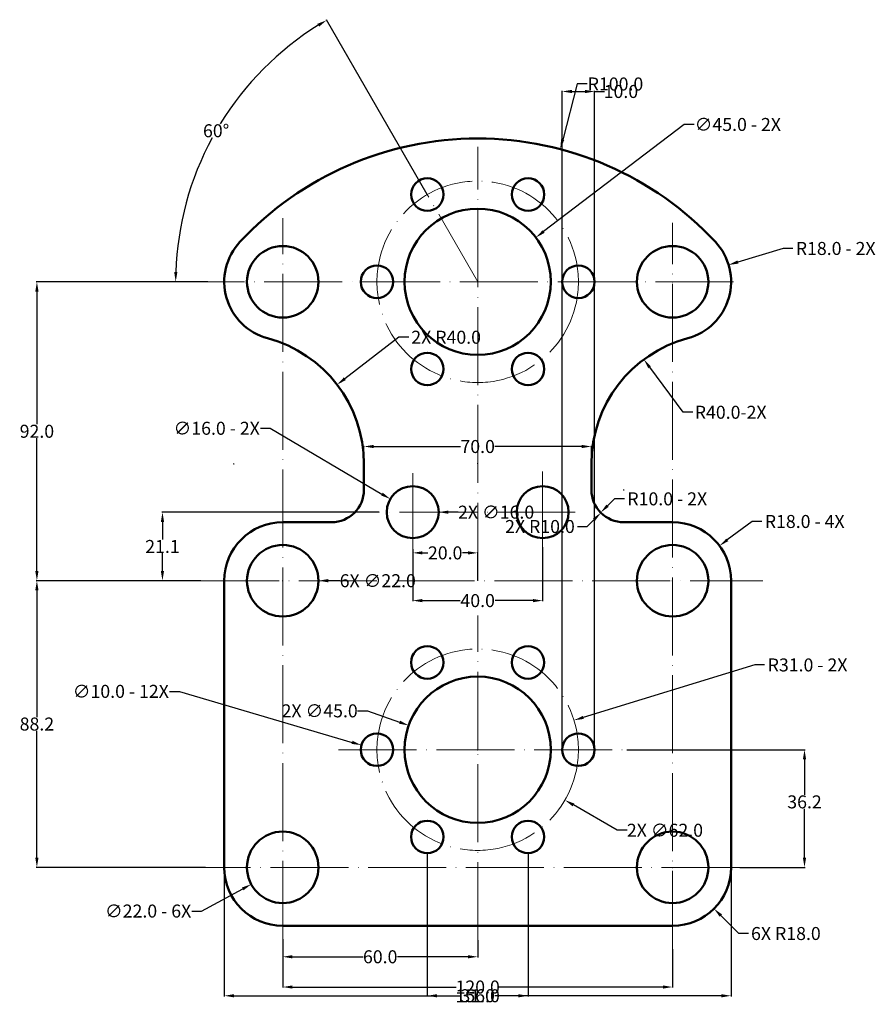
# Model space of a CAD drawing. Units: inches. Extents: x 135 to 399, y 77 to 380.
import ezdxf

# ---------------------------------------------------------------- set-up
doc = ezdxf.new("R2010")
doc.units = ezdxf.units.IN
doc.header["$MEASUREMENT"] = 0
doc.linetypes.add('ACAD_ISO04W100', pattern=[30, 24, -3, 0, -3])
for name, color, linetype, lineweight in [('M-CNTR', 4, 'ACAD_ISO04W100', 18), ('M-DIMS', 2, 'Continuous', 25), ('M-OUTL', 7, 'Continuous', 50)]:
    doc.layers.add(name, color=color, linetype=linetype, lineweight=lineweight)
doc.styles.get("Standard").update_dxf_attribs({"font": 'arial.ttf'})
doc.dimstyles.get("Standard").update_dxf_attribs({"dimtxt": 4, "dimasz": 3, "dimexe": 0.18, "dimexo": 0.0625, "dimgap": 0.09, "dimtad": 0, "dimtih": 1, "dimtoh": 1, "dimdec": 1, "dimzin": 0, "dimdsep": 46, "dimtxsty": 'Standard', "dimcen": 0.09, "dimclrd": 1, "dimclre": 1, "dimadec": 0, "dimazin": 0, "dimtfac": 1, "dimtdec": 1, "dimtofl": 0, "dimtmove": 0, "dimatfit": 3, "dimfxl": 1, "dimtolj": 1, "dimtzin": 0, "dimarcsym": 0})

# ---------------------------------------------------------------- blocks, each defined once
blk = doc.blocks.new('*U1')
blk.add_circle((0, 0), 5)
blk = doc.blocks.new('*U2')
at = {"layer": 'M-OUTL', "color": 0, "linetype": 'ByBlock', "lineweight": -2, "transparency": 16777216}
for p, rotation in [((163.06, 105.92), 120), ((194.06, 105.92), 59.99999999999999), ((147.56, 79.07), 180), ((163.06, 52.23), 239.9999999999999), ((194.06, 52.23), 299.9999999999999)]:
    blk.add_blockref('*U1', p, dxfattribs=dict(at, rotation=rotation))
blk.add_blockref('*U1', (209.56, 79.07), dxfattribs=at)
blk = doc.blocks.new('*D3')
at = {"layer": 'Defpoints', "color": 0, "transparency": 16777216}
for p in [(322.16, 155.02), (356.94, 118.82), (376.93, 118.82)]:
    blk.add_point(p, dxfattribs=at)
at = {"layer": 'M-DIMS', "color": 0, "lineweight": -2, "transparency": 16777216}
for p, q in [((322.22, 155.02), (377.11, 155.02)), ((376.93, 152.02), (376.93, 141.1)), ((376.93, 121.82), (376.93, 136.83)), ((357, 118.82), (377.11, 118.82))]:
    blk.add_line(p, q, dxfattribs=at)
at = {"layer": 'M-DIMS', "color": 0, "transparency": 16777216}
for points in [[(376.43, 152.02), (377.43, 152.02), (376.93, 155.02)], [(376.43, 121.82), (377.43, 121.82), (376.93, 118.82)]]:
    blk.add_solid(points, dxfattribs=at)
at = {"layer": 'M-DIMS', "color": 0, "transparency": 16777216, "insert": (376.93, 138.97), "char_height": 4, "attachment_point": 5}
blk.add_mtext('\\A1;36.2', dxfattribs=at)
blk = doc.blocks.new('*D4')
at = {"layer": 'Defpoints', "color": 0, "transparency": 16777216}
for p in [(216.34, 96.82), (276.34, 96.43), (216.34, 91.3)]:
    blk.add_point(p, dxfattribs=at)
at = {"layer": 'M-DIMS', "color": 0, "lineweight": -2, "transparency": 16777216}
for p, q in [((216.34, 96.76), (216.34, 91.12)), ((276.34, 96.37), (276.34, 91.12)), ((219.34, 91.3), (241.05, 91.3)), ((273.34, 91.3), (251.63, 91.3))]:
    blk.add_line(p, q, dxfattribs=at)
at = {"layer": 'M-DIMS', "color": 0, "transparency": 16777216}
for points in [[(219.34, 91.8), (219.34, 90.8), (216.34, 91.3)], [(273.34, 91.8), (273.34, 90.8), (276.34, 91.3)]]:
    blk.add_solid(points, dxfattribs=at)
at = {"layer": 'M-DIMS', "color": 0, "transparency": 16777216, "insert": (246.34, 91.3), "char_height": 4, "attachment_point": 5}
blk.add_mtext('\\A1;60.0', dxfattribs=at)
blk = doc.blocks.new('*D5')
at = {"layer": 'Defpoints', "color": 0, "transparency": 16777216}
for p in [(216.34, 96.82), (336.34, 93.75), (216.34, 81.99)]:
    blk.add_point(p, dxfattribs=at)
at = {"layer": 'M-DIMS', "color": 0, "lineweight": -2, "transparency": 16777216}
for p, q in [((216.34, 96.76), (216.34, 81.81)), ((336.34, 93.68), (336.34, 81.81)), ((219.34, 81.99), (269.69, 81.99)), ((333.34, 81.99), (282.98, 81.99))]:
    blk.add_line(p, q, dxfattribs=at)
at = {"layer": 'M-DIMS', "color": 0, "transparency": 16777216}
for points in [[(219.34, 82.49), (219.34, 81.49), (216.34, 81.99)], [(333.34, 82.49), (333.34, 81.49), (336.34, 81.99)]]:
    blk.add_solid(points, dxfattribs=at)
at = {"layer": 'M-DIMS', "color": 0, "transparency": 16777216, "insert": (276.34, 81.99), "char_height": 4, "attachment_point": 5}
blk.add_mtext('\\A1;120.0', dxfattribs=at)
blk = doc.blocks.new('*D6')
at = {"layer": 'Defpoints', "color": 0, "transparency": 16777216}
for p in [(226.02, 124.04), (206.65, 113.61)]:
    blk.add_point(p, dxfattribs=at)
at = {"layer": 'M-DIMS', "color": 0, "lineweight": -2, "transparency": 16777216}
for p, q in [((216.25, 118.82), (216.43, 118.82)), ((216.34, 118.73), (216.34, 118.91)), ((191.38, 105.37), (204.01, 112.18)), ((188.38, 105.37), (191.38, 105.37))]:
    blk.add_line(p, q, dxfattribs=at)
at = {"layer": 'M-DIMS', "color": 0, "transparency": 16777216}
blk.add_solid([(203.78, 112.62), (204.25, 111.74), (206.65, 113.61)], dxfattribs=at)
at = {"layer": 'M-DIMS', "color": 0, "transparency": 16777216, "insert": (174.91, 105.37), "char_height": 4, "attachment_point": 5}
blk.add_mtext('\\A1;∅22.0 - 6X', dxfattribs=at)
blk = doc.blocks.new('*D7')
at = {"layer": 'Defpoints', "color": 0, "transparency": 16777216}
for p in [(305.98, 164.09), (276.34, 155.02)]:
    blk.add_point(p, dxfattribs=at)
at = {"layer": 'M-DIMS', "color": 0, "lineweight": -2, "transparency": 16777216}
for p, q in [((361.66, 181.11), (308.85, 164.97)), ((364.66, 181.11), (361.66, 181.11)), ((276.25, 155.02), (276.43, 155.02)), ((276.34, 154.93), (276.34, 155.11))]:
    blk.add_line(p, q, dxfattribs=at)
at = {"layer": 'M-DIMS', "color": 0, "transparency": 16777216}
blk.add_solid([(308.71, 165.44), (309, 164.49), (305.98, 164.09)], dxfattribs=at)
at = {"layer": 'M-DIMS', "color": 0, "transparency": 16777216, "insert": (377.87, 181.11), "char_height": 4, "attachment_point": 5}
blk.add_mtext('\\A1;R31.0 - 2X', dxfattribs=at)
blk = doc.blocks.new('*D8')
at = {"layer": 'Defpoints', "color": 0, "transparency": 16777216}
for p in [(240.54, 156.44), (250.13, 153.61)]:
    blk.add_point(p, dxfattribs=at)
at = {"layer": 'M-DIMS', "color": 0, "lineweight": -2, "transparency": 16777216}
for p, q in [((181.54, 172.98), (184.54, 172.98)), ((184.54, 172.98), (237.67, 157.29)), ((245.25, 155.02), (245.43, 155.02)), ((245.34, 154.93), (245.34, 155.11))]:
    blk.add_line(p, q, dxfattribs=at)
at = {"layer": 'M-DIMS', "color": 0, "transparency": 16777216}
blk.add_solid([(237.81, 157.77), (237.52, 156.81), (240.54, 156.44)], dxfattribs=at)
at = {"layer": 'M-DIMS', "color": 0, "transparency": 16777216, "insert": (166.51, 172.98), "char_height": 4, "attachment_point": 5}
blk.add_mtext('\\A1;∅10.0 - 12X', dxfattribs=at)
blk = doc.blocks.new('*D9')
at = {"layer": 'Defpoints', "color": 0, "transparency": 16777216}
for p in [(191.21, 207.02), (140.68, 118.82), (192.68, 118.82)]:
    blk.add_point(p, dxfattribs=at)
at = {"layer": 'M-DIMS', "color": 0, "lineweight": -2, "transparency": 16777216}
for p, q in [((191.15, 207.02), (140.5, 207.02)), ((140.68, 204.02), (140.68, 165.06)), ((140.68, 121.82), (140.68, 160.79)), ((192.62, 118.82), (140.5, 118.82))]:
    blk.add_line(p, q, dxfattribs=at)
at = {"layer": 'M-DIMS', "color": 0, "transparency": 16777216}
for points in [[(140.18, 204.02), (141.18, 204.02), (140.68, 207.02)], [(140.18, 121.82), (141.18, 121.82), (140.68, 118.82)]]:
    blk.add_solid(points, dxfattribs=at)
at = {"layer": 'M-DIMS', "color": 0, "transparency": 16777216, "insert": (140.68, 162.92), "char_height": 4, "attachment_point": 5}
blk.add_mtext('\\A1;88.2', dxfattribs=at)
blk = doc.blocks.new('*D10')
at = {"layer": 'Defpoints', "color": 0, "transparency": 16777216}
for p in [(179.32, 228.12), (246.09, 228.12), (191.21, 207.02)]:
    blk.add_point(p, dxfattribs=at)
at = {"layer": 'M-DIMS', "color": 0, "lineweight": -2, "transparency": 16777216}
for p, q in [((246.02, 228.12), (179.14, 228.12)), ((179.32, 225.12), (179.32, 219.67)), ((179.32, 210.02), (179.32, 215.48)), ((191.15, 207.02), (179.14, 207.02))]:
    blk.add_line(p, q, dxfattribs=at)
at = {"layer": 'M-DIMS', "color": 0, "transparency": 16777216}
for points in [[(178.82, 225.12), (179.82, 225.12), (179.32, 228.12)], [(178.82, 210.02), (179.82, 210.02), (179.32, 207.02)]]:
    blk.add_solid(points, dxfattribs=at)
at = {"layer": 'M-DIMS', "color": 0, "transparency": 16777216, "insert": (179.32, 217.57), "char_height": 4, "attachment_point": 5}
blk.add_mtext('\\A1;21.1', dxfattribs=at)
blk = doc.blocks.new('*D11')
at = {"layer": 'Defpoints', "color": 0, "transparency": 16777216}
for p in [(256.34, 216.79), (296.34, 217.44), (296.34, 200.91)]:
    blk.add_point(p, dxfattribs=at)
at = {"layer": 'M-DIMS', "color": 0, "lineweight": -2, "transparency": 16777216}
for p, q in [((256.34, 216.73), (256.34, 200.73)), ((296.34, 217.38), (296.34, 200.73)), ((259.34, 200.91), (270.98, 200.91)), ((293.34, 200.91), (281.7, 200.91))]:
    blk.add_line(p, q, dxfattribs=at)
at = {"layer": 'M-DIMS', "color": 0, "transparency": 16777216}
for points in [[(259.34, 201.41), (259.34, 200.41), (256.34, 200.91)], [(293.34, 201.41), (293.34, 200.41), (296.34, 200.91)]]:
    blk.add_solid(points, dxfattribs=at)
at = {"layer": 'M-DIMS', "color": 0, "transparency": 16777216, "insert": (276.34, 200.91), "char_height": 4, "attachment_point": 5}
blk.add_mtext('\\A1;40.0', dxfattribs=at)
blk = doc.blocks.new('*D12')
at = {"layer": 'Defpoints', "color": 0, "transparency": 16777216}
for p in [(249.44, 232.18), (263.23, 224.07)]:
    blk.add_point(p, dxfattribs=at)
at = {"layer": 'M-DIMS', "color": 0, "lineweight": -2, "transparency": 16777216}
for p, q in [((209.49, 253.94), (212.49, 253.94)), ((212.49, 253.94), (246.86, 233.71)), ((256.25, 228.12), (256.43, 228.12)), ((256.34, 228.03), (256.34, 228.21))]:
    blk.add_line(p, q, dxfattribs=at)
at = {"layer": 'M-DIMS', "color": 0, "transparency": 16777216}
blk.add_solid([(247.11, 234.14), (246.6, 233.27), (249.44, 232.18)], dxfattribs=at)
at = {"layer": 'M-DIMS', "color": 0, "transparency": 16777216, "insert": (196.02, 253.94), "char_height": 4, "attachment_point": 5}
blk.add_mtext('\\A1;∅16.0 - 2X', dxfattribs=at)
blk = doc.blocks.new('*D13')
at = {"layer": 'Defpoints', "color": 0, "transparency": 16777216}
for p in [(256.34, 216.79), (276.34, 215.6), (276.34, 207.02)]:
    blk.add_point(p, dxfattribs=at)
at = {"layer": 'M-DIMS', "color": 0, "lineweight": -2, "transparency": 16777216}
for p, q in [((256.34, 216.73), (256.34, 215.42)), ((259.34, 215.6), (261.03, 215.6)), ((273.34, 215.6), (271.65, 215.6)), ((276.34, 207.09), (276.34, 215.78))]:
    blk.add_line(p, q, dxfattribs=at)
at = {"layer": 'M-DIMS', "color": 0, "transparency": 16777216}
for points in [[(259.34, 216.1), (259.34, 215.1), (256.34, 215.6)], [(273.34, 216.1), (273.34, 215.1), (276.34, 215.6)]]:
    blk.add_solid(points, dxfattribs=at)
at = {"layer": 'M-DIMS', "color": 0, "transparency": 16777216, "insert": (266.34, 215.6), "char_height": 4, "attachment_point": 5}
blk.add_mtext('\\A1;20.0', dxfattribs=at)
blk = doc.blocks.new('*U14')
blk.add_circle((0, 0), 5)
blk = doc.blocks.new('*U15')
at = {"layer": 'M-OUTL', "color": 0, "linetype": 'ByBlock', "lineweight": -2, "transparency": 16777216}
for p, rotation in [((260.84, 325.87), 120), ((291.84, 325.87), 59.99999999999999), ((245.34, 299.02), 180), ((260.84, 272.18), 239.9999999999999), ((291.84, 272.18), 299.9999999999999)]:
    blk.add_blockref('*U14', p, dxfattribs=dict(at, rotation=rotation))
blk.add_blockref('*U14', (307.34, 299.02), dxfattribs=at)
blk = doc.blocks.new('*D16')
at = {"layer": 'Defpoints', "color": 0, "transparency": 16777216}
for p in [(205.13, 358.77), (260.84, 325.87), (193.34, 299.02), (276.34, 299.02), (355.06, 299.02)]:
    blk.add_point(p, dxfattribs=at)
at = {"layer": 'M-DIMS', "color": 0, "lineweight": -2, "transparency": 16777216}
for p, q in [((260.81, 325.93), (229.77, 379.68)), ((193.27, 299.02), (183.21, 299.02))]:
    blk.add_line(p, q, dxfattribs=at)
for start, end in [(121.8493, 148.4703), (151.5064, 178.1507)]:
    blk.add_arc((276.34, 299.02), 92.95, start, end, dxfattribs=at)
at = {"layer": 'M-DIMS', "color": 0, "transparency": 16777216}
for points in [[(227.03, 378.41), (227.55, 377.55), (229.86, 379.52)], [(183.93, 302.02), (182.94, 302.03), (183.39, 299.02)]]:
    blk.add_solid(points, dxfattribs=at)
at = {"layer": 'M-DIMS', "color": 0, "transparency": 16777216, "insert": (195.84, 345.5), "char_height": 4, "attachment_point": 5}
blk.add_mtext('\\A1;60°', dxfattribs=at)
blk = doc.blocks.new('*D17')
at = {"layer": 'Defpoints', "color": 0, "transparency": 16777216}
for p in [(301.74, 339.85), (276.34, 243.13)]:
    blk.add_point(p, dxfattribs=at)
at = {"layer": 'M-DIMS', "color": 0, "lineweight": -2, "transparency": 16777216}
for p, q in [((307.01, 359.89), (302.51, 342.75)), ((310.01, 359.89), (307.01, 359.89)), ((276.25, 243.13), (276.43, 243.13)), ((276.34, 243.04), (276.34, 243.22))]:
    blk.add_line(p, q, dxfattribs=at)
at = {"layer": 'M-DIMS', "color": 0, "transparency": 16777216}
blk.add_solid([(302.02, 342.88), (302.99, 342.63), (301.74, 339.85)], dxfattribs=at)
at = {"layer": 'M-DIMS', "color": 0, "transparency": 16777216, "insert": (318.75, 359.89), "char_height": 4, "attachment_point": 5}
blk.add_mtext('\\A1;R100.0', dxfattribs=at)
blk = doc.blocks.new('*D18')
at = {"layer": 'Defpoints', "color": 0, "transparency": 16777216}
for p in [(294.24, 312.65), (258.44, 285.4)]:
    blk.add_point(p, dxfattribs=at)
at = {"layer": 'M-DIMS', "color": 0, "lineweight": -2, "transparency": 16777216}
for p, q in [((339.94, 347.44), (296.63, 314.47)), ((342.94, 347.44), (339.94, 347.44)), ((276.25, 299.02), (276.43, 299.02)), ((276.34, 298.93), (276.34, 299.11))]:
    blk.add_line(p, q, dxfattribs=at)
at = {"layer": 'M-DIMS', "color": 0, "transparency": 16777216}
blk.add_solid([(296.32, 314.87), (296.93, 314.07), (294.24, 312.65)], dxfattribs=at)
at = {"layer": 'M-DIMS', "color": 0, "transparency": 16777216, "insert": (356.41, 347.44), "char_height": 4, "attachment_point": 5}
blk.add_mtext('\\A1;∅45.0 - 2X', dxfattribs=at)
blk = doc.blocks.new('*D19')
at = {"layer": 'Defpoints', "color": 0, "transparency": 16777216}
for p in [(353.57, 304.22), (336.34, 299.02)]:
    blk.add_point(p, dxfattribs=at)
at = {"layer": 'M-DIMS', "color": 0, "lineweight": -2, "transparency": 16777216}
for p, q in [((370.32, 309.28), (356.44, 305.09)), ((373.32, 309.28), (370.32, 309.28)), ((336.25, 299.02), (336.43, 299.02)), ((336.34, 298.93), (336.34, 299.11))]:
    blk.add_line(p, q, dxfattribs=at)
at = {"layer": 'M-DIMS', "color": 0, "transparency": 16777216}
blk.add_solid([(356.3, 305.57), (356.59, 304.61), (353.57, 304.22)], dxfattribs=at)
at = {"layer": 'M-DIMS', "color": 0, "transparency": 16777216, "insert": (386.53, 309.28), "char_height": 4, "attachment_point": 5}
blk.add_mtext('\\A1;R18.0 - 2X', dxfattribs=at)
blk = doc.blocks.new('*D20')
at = {"layer": 'Defpoints', "color": 0, "transparency": 16777216}
for p in [(327.49, 275.11), (351.34, 243)]:
    blk.add_point(p, dxfattribs=at)
at = {"layer": 'M-DIMS', "color": 0, "lineweight": -2, "transparency": 16777216}
for p, q in [((339.55, 258.87), (329.28, 272.71)), ((342.55, 258.87), (339.55, 258.87))]:
    blk.add_line(p, q, dxfattribs=at)
at = {"layer": 'M-DIMS', "color": 0, "transparency": 16777216}
blk.add_solid([(329.68, 273), (328.88, 272.41), (327.49, 275.11)], dxfattribs=at)
at = {"layer": 'M-DIMS', "color": 0, "transparency": 16777216, "insert": (354.21, 258.87), "char_height": 4, "attachment_point": 5}
blk.add_mtext('\\A1;R40.0-2X', dxfattribs=at)
blk = doc.blocks.new('*D21')
at = {"layer": 'Defpoints', "color": 0, "transparency": 16777216}
for p in [(311.34, 248.33), (241.34, 239.01), (311.34, 239.01)]:
    blk.add_point(p, dxfattribs=at)
at = {"layer": 'M-DIMS', "color": 0, "lineweight": -2, "transparency": 16777216}
for p, q in [((241.34, 239.07), (241.34, 248.51)), ((311.34, 239.07), (311.34, 248.51)), ((244.34, 248.33), (271.08, 248.33)), ((308.34, 248.33), (281.6, 248.33))]:
    blk.add_line(p, q, dxfattribs=at)
at = {"layer": 'M-DIMS', "color": 0, "transparency": 16777216}
for points in [[(244.34, 248.83), (244.34, 247.83), (241.34, 248.33)], [(308.34, 248.83), (308.34, 247.83), (311.34, 248.33)]]:
    blk.add_solid(points, dxfattribs=at)
at = {"layer": 'M-DIMS', "color": 0, "transparency": 16777216, "insert": (276.34, 248.33), "char_height": 4, "attachment_point": 5}
blk.add_mtext('\\A1;70.0', dxfattribs=at)
blk = doc.blocks.new('*D22')
at = {"layer": 'Defpoints', "color": 0, "transparency": 16777216}
for p in [(321.34, 235.02), (314.2, 228.02)]:
    blk.add_point(p, dxfattribs=at)
at = {"layer": 'M-DIMS', "color": 0, "lineweight": -2, "transparency": 16777216}
for p, q in [((318.48, 232.22), (316.34, 230.12)), ((321.48, 232.22), (318.48, 232.22))]:
    blk.add_line(p, q, dxfattribs=at)
at = {"layer": 'M-DIMS', "color": 0, "transparency": 16777216}
blk.add_solid([(315.99, 230.48), (316.69, 229.77), (314.2, 228.02)], dxfattribs=at)
at = {"layer": 'M-DIMS', "color": 0, "transparency": 16777216, "insert": (334.69, 232.22), "char_height": 4, "attachment_point": 5}
blk.add_mtext('\\A1;R10.0 - 2X', dxfattribs=at)
blk = doc.blocks.new('*D23')
at = {"layer": 'Defpoints', "color": 0, "transparency": 16777216}
for p in [(350.76, 217.79), (336.34, 207.02)]:
    blk.add_point(p, dxfattribs=at)
at = {"layer": 'M-DIMS', "color": 0, "lineweight": -2, "transparency": 16777216}
for p, q in [((360.78, 225.26), (353.17, 219.58)), ((363.78, 225.26), (360.78, 225.26)), ((336.25, 207.02), (336.43, 207.02)), ((336.34, 206.93), (336.34, 207.11))]:
    blk.add_line(p, q, dxfattribs=at)
at = {"layer": 'M-DIMS', "color": 0, "transparency": 16777216}
blk.add_solid([(352.87, 219.98), (353.47, 219.18), (350.76, 217.79)], dxfattribs=at)
at = {"layer": 'M-DIMS', "color": 0, "transparency": 16777216, "insert": (376.99, 225.26), "char_height": 4, "attachment_point": 5}
blk.add_mtext('\\A1;R18.0 - 4X', dxfattribs=at)
blk = doc.blocks.new('*D24')
at = {"layer": 'Defpoints', "color": 0, "transparency": 16777216}
for p in [(193.34, 299.02), (140.68, 207.02), (191.21, 207.02)]:
    blk.add_point(p, dxfattribs=at)
at = {"layer": 'M-DIMS', "color": 0, "lineweight": -2, "transparency": 16777216}
for p, q in [((193.27, 299.02), (140.5, 299.02)), ((140.68, 296.02), (140.68, 255.16)), ((140.68, 210.02), (140.68, 250.89)), ((191.15, 207.02), (140.5, 207.02))]:
    blk.add_line(p, q, dxfattribs=at)
at = {"layer": 'M-DIMS', "color": 0, "transparency": 16777216}
for points in [[(140.18, 296.02), (141.18, 296.02), (140.68, 299.02)], [(140.18, 210.02), (141.18, 210.02), (140.68, 207.02)]]:
    blk.add_solid(points, dxfattribs=at)
at = {"layer": 'M-DIMS', "color": 0, "transparency": 16777216, "insert": (140.68, 253.02), "char_height": 4, "attachment_point": 5}
blk.add_mtext('\\A1;92.0', dxfattribs=at)
blk = doc.blocks.new('*D25')
at = {"layer": 'Defpoints', "color": 0, "transparency": 16777216}
for p in [(198.34, 207.02), (354.34, 207.02), (354.34, 79.3)]:
    blk.add_point(p, dxfattribs=at)
at = {"layer": 'M-DIMS', "color": 1, "lineweight": -2, "transparency": 16777216}
for p, q in [((198.34, 206.96), (198.34, 79.12)), ((354.34, 206.96), (354.34, 79.12)), ((201.34, 79.3), (269.69, 79.3)), ((351.34, 79.3), (282.98, 79.3))]:
    blk.add_line(p, q, dxfattribs=at)
at = {"layer": 'M-DIMS', "color": 1, "transparency": 16777216}
for points in [[(201.34, 79.8), (201.34, 78.8), (198.34, 79.3)], [(351.34, 79.8), (351.34, 78.8), (354.34, 79.3)]]:
    blk.add_solid(points, dxfattribs=at)
at = {"layer": 'M-DIMS', "color": 0, "transparency": 16777216, "insert": (276.34, 79.3), "char_height": 4, "attachment_point": 5}
blk.add_mtext('\\A1;156.0', dxfattribs=at)
blk = doc.blocks.new('*D26')
at = {"layer": 'Defpoints', "color": 0, "transparency": 16777216}
for p in [(312.337582, 357.581874), (302.337582, 155.024628), (312.337582, 155.024628)]:
    blk.add_point(p, dxfattribs=at)
at = {"layer": 'M-DIMS', "color": 1, "lineweight": -2, "transparency": 16777216}
for p, q in [((302.337582, 155.087128), (302.337582, 357.761874)), ((305.337582, 357.581874), (309.337582, 357.581874)), ((312.337582, 155.087128), (312.337582, 357.761874)), ((312.337582, 357.581874), (315.337582, 357.581874))]:
    blk.add_line(p, q, dxfattribs=at)
at = {"layer": 'M-DIMS', "color": 1, "transparency": 16777216}
for points in [[(305.337582, 358.081874), (305.337582, 357.081874), (302.337582, 357.581874)], [(309.337582, 358.081874), (309.337582, 357.081874), (312.337582, 357.581874)]]:
    blk.add_solid(points, dxfattribs=at)
at = {"layer": 'M-DIMS', "color": 0, "transparency": 16777216, "insert": (320.427582, 357.581874), "char_height": 4, "attachment_point": 5}
blk.add_mtext('\\A1;10.0', dxfattribs=at)
blk = doc.blocks.new('*D27')
at = {"layer": 'Defpoints', "color": 0, "transparency": 16777216}
for p in [(260.84, 123.18), (291.84, 123.18), (291.84, 79.3)]:
    blk.add_point(p, dxfattribs=at)
at = {"layer": 'M-DIMS', "color": 1, "lineweight": -2, "transparency": 16777216}
for p, q in [((260.84, 123.12), (260.84, 79.12)), ((291.84, 123.12), (291.84, 79.12)), ((263.84, 79.3), (271.06, 79.3)), ((288.84, 79.3), (281.61, 79.3))]:
    blk.add_line(p, q, dxfattribs=at)
at = {"layer": 'M-DIMS', "color": 1, "transparency": 16777216}
for points in [[(263.84, 79.8), (263.84, 78.8), (260.84, 79.3)], [(288.84, 79.8), (288.84, 78.8), (291.84, 79.3)]]:
    blk.add_solid(points, dxfattribs=at)
at = {"layer": 'M-DIMS', "color": 0, "transparency": 16777216, "insert": (276.34, 79.3), "char_height": 4, "attachment_point": 5}
blk.add_mtext('\\A1;31.0', dxfattribs=at)
blk = doc.blocks.new('*D28')
at = {"layer": 'Defpoints', "color": 0, "transparency": 16777216}
for p in [(233.07, 267.35), (201.34, 243)]:
    blk.add_point(p, dxfattribs=at)
at = {"layer": 'M-DIMS', "color": 1, "lineweight": -2, "transparency": 16777216}
for p, q in [((252.11, 281.96), (235.45, 269.18)), ((255.11, 281.96), (252.11, 281.96)), ((201.25, 243), (201.43, 243)), ((201.34, 242.91), (201.34, 243.09))]:
    blk.add_line(p, q, dxfattribs=at)
at = {"layer": 'M-DIMS', "color": 1, "transparency": 16777216}
blk.add_solid([(235.14, 269.58), (235.75, 268.78), (233.07, 267.35)], dxfattribs=at)
at = {"layer": 'M-DIMS', "color": 0, "transparency": 16777216, "insert": (266.63, 281.96), "char_height": 4, "attachment_point": 5}
blk.add_mtext('\\A1;2X R40.0', dxfattribs=at)
blk = doc.blocks.new('*D29')
at = {"layer": 'Defpoints', "color": 0, "transparency": 16777216}
for p in [(249.49, 170.52), (303.19, 139.53)]:
    blk.add_point(p, dxfattribs=at)
at = {"layer": 'M-DIMS', "color": 1, "lineweight": -2, "transparency": 16777216}
for p, q in [((276.25, 155.02), (276.43, 155.02)), ((276.34, 154.93), (276.34, 155.11)), ((319.3, 130.24), (305.79, 138.03)), ((322.3, 130.24), (319.3, 130.24))]:
    blk.add_line(p, q, dxfattribs=at)
at = {"layer": 'M-DIMS', "color": 1, "transparency": 16777216}
blk.add_solid([(306.04, 138.47), (305.54, 137.6), (303.19, 139.53)], dxfattribs=at)
at = {"layer": 'M-DIMS', "color": 0, "transparency": 16777216, "insert": (333.98, 130.24), "char_height": 4, "attachment_point": 5}
blk.add_mtext('\\A1;2X ∅62.0', dxfattribs=at)
blk = doc.blocks.new('*D30')
at = {"layer": 'Defpoints', "color": 0, "transparency": 16777216}
for p in [(255.11, 162.5), (297.56, 147.55)]:
    blk.add_point(p, dxfattribs=at)
at = {"layer": 'M-DIMS', "color": 1, "lineweight": -2, "transparency": 16777216}
for p, q in [((239.38, 166.98), (242.38, 166.98)), ((242.38, 166.98), (252.28, 163.49)), ((276.25, 155.02), (276.43, 155.02)), ((276.34, 154.93), (276.34, 155.11))]:
    blk.add_line(p, q, dxfattribs=at)
at = {"layer": 'M-DIMS', "color": 1, "transparency": 16777216}
blk.add_solid([(252.45, 163.96), (252.12, 163.02), (255.11, 162.5)], dxfattribs=at)
at = {"layer": 'M-DIMS', "color": 0, "transparency": 16777216, "insert": (227.7, 166.98), "char_height": 4, "attachment_point": 5}
blk.add_mtext('\\A1;2X ∅45.0', dxfattribs=at)
blk = doc.blocks.new('*D31')
at = {"layer": 'Defpoints', "color": 0, "transparency": 16777216}
for p in [(336.34, 118.82), (349.07, 106.1)]:
    blk.add_point(p, dxfattribs=at)
at = {"layer": 'M-DIMS', "color": 1, "lineweight": -2, "transparency": 16777216}
for p, q in [((336.25, 118.82), (336.43, 118.82)), ((336.34, 118.73), (336.34, 118.91)), ((356.7, 98.46), (351.19, 103.98)), ((359.7, 98.46), (356.7, 98.46))]:
    blk.add_line(p, q, dxfattribs=at)
at = {"layer": 'M-DIMS', "color": 1, "transparency": 16777216}
blk.add_solid([(351.54, 104.33), (350.83, 103.62), (349.07, 106.1)], dxfattribs=at)
at = {"layer": 'M-DIMS', "color": 0, "transparency": 16777216, "insert": (371.2, 98.46), "char_height": 4, "attachment_point": 5}
blk.add_mtext('\\A1;6X R18.0', dxfattribs=at)
blk = doc.blocks.new('*D32')
at = {"layer": 'Defpoints', "color": 0, "transparency": 16777216}
for p in [(205.34, 207.02), (227.34, 207.03)]:
    blk.add_point(p, dxfattribs=at)
at = {"layer": 'M-DIMS', "color": 1, "lineweight": -2, "transparency": 16777216}
for p, q in [((216.25, 207.02), (216.43, 207.02)), ((216.34, 206.93), (216.34, 207.11)), ((233.94, 207.03), (230.34, 207.03))]:
    blk.add_line(p, q, dxfattribs=at)
at = {"layer": 'M-DIMS', "color": 1, "transparency": 16777216}
blk.add_solid([(230.34, 207.53), (230.34, 206.53), (227.34, 207.03)], dxfattribs=at)
at = {"layer": 'M-DIMS', "color": 0, "transparency": 16777216, "insert": (245.59, 207.03), "char_height": 4, "attachment_point": 5}
blk.add_mtext('\\A1;6X ∅22.0', dxfattribs=at)
blk = doc.blocks.new('*D33')
at = {"layer": 'Defpoints', "color": 0, "transparency": 16777216}
for p in [(321.34, 235.02), (314.27, 227.95)]:
    blk.add_point(p, dxfattribs=at)
at = {"layer": 'M-DIMS', "color": 1, "lineweight": -2, "transparency": 16777216}
for p, q in [((321.25, 235.02), (321.43, 235.02)), ((321.34, 234.93), (321.34, 235.11)), ((310.02, 223.71), (312.15, 225.83)), ((307.02, 223.71), (310.02, 223.71))]:
    blk.add_line(p, q, dxfattribs=at)
at = {"layer": 'M-DIMS', "color": 1, "transparency": 16777216}
blk.add_solid([(311.79, 226.19), (312.5, 225.48), (314.27, 227.95)], dxfattribs=at)
at = {"layer": 'M-DIMS', "color": 0, "transparency": 16777216, "insert": (295.5, 223.71), "char_height": 4, "attachment_point": 5}
blk.add_mtext('\\A1;2X R10.0', dxfattribs=at)
blk = doc.blocks.new('*D34')
at = {"layer": 'Defpoints', "color": 0, "transparency": 16777216}
for p in [(248.34, 228.12), (264.34, 228.12)]:
    blk.add_point(p, dxfattribs=at)
at = {"layer": 'M-DIMS', "color": 1, "lineweight": -2, "transparency": 16777216}
for p, q in [((256.25, 228.12), (256.43, 228.12)), ((256.34, 228.03), (256.34, 228.21)), ((270.34, 228.13), (267.34, 228.13))]:
    blk.add_line(p, q, dxfattribs=at)
at = {"layer": 'M-DIMS', "color": 1, "transparency": 16777216}
blk.add_solid([(267.34, 228.63), (267.34, 227.63), (264.34, 228.12)], dxfattribs=at)
at = {"layer": 'M-DIMS', "color": 0, "transparency": 16777216, "insert": (282.02, 228.13), "char_height": 4, "attachment_point": 5}
blk.add_mtext('\\A1;2X ∅16.0', dxfattribs=at)

msp = doc.modelspace()

# ---------------------------------------------------------------- linework, layer by layer
at = {"layer": 'M-CNTR'}
for p, q in [((276.34, 207.02), (276.34, 340.53)), ((276.34, 299.02), (260.84, 325.87)), ((216.34, 96.82), (216.34, 318.58)), ((336.34, 93.75), (336.34, 317.14)), ((355.06, 299.02), (193.34, 299.02)), ((256.34, 240.08), (256.34, 216.79)), ((296.34, 240.61), (296.34, 217.44)), ((306.35, 228.12), (246.09, 228.12)), ((191.21, 207.02), (364.15, 207.02)), ((276.34, 155.02), (276.34, 196.3)), ((233.53, 155.02), (322.16, 155.02)), ((276.34, 96.43), (276.34, 155.02)), ((356.94, 118.82), (192.68, 118.82))]:
    msp.add_line(p, q, dxfattribs=at)
for centre in [(276.34, 299.02), (276.34, 155.02)]:
    msp.add_circle(centre, 31, dxfattribs=at)
at = {"layer": 'M-OUTL'}
for p, q in [((241.34, 235.02), (241.34, 243)), ((311.34, 235.02), (311.34, 243)), ((216.34, 225.02), (231.34, 225.02)), ((321.34, 225.02), (336.34, 225.02)), ((198.34, 118.82), (198.34, 207.02)), ((354.34, 118.82), (354.34, 207.02)), ((216.34, 100.82), (336.34, 100.82))]:
    msp.add_line(p, q, dxfattribs=at)
for centre, radius in [((276.34, 299.02), 22.5), ((216.34, 299.02), 11), ((336.34, 299.02), 11), ((256.34, 228.12), 8), ((296.34, 228.12), 8), ((216.34, 207.02), 11), ((336.34, 207.02), 11), ((276.34, 155.02), 22.5), ((216.34, 118.82), 11), ((336.34, 118.82), 11)]:
    msp.add_circle(centre, radius, dxfattribs=at)
for centre, radius, start, end in [((276.34, 243.13), 100, 42.9703, 137.0297), ((216.34, 299.02), 18, 137.0297, 255.0118), ((336.34, 299.02), 18, 284.9882, 42.9703), ((201.34, 243), 40, 0, 75.0118), ((351.34, 243), 40, 104.9882, 180), ((231.34, 235.02), 10, 270, 0), ((321.34, 235.02), 10, 180, 270), ((216.34, 207.02), 18, 90, 180), ((336.34, 207.02), 18, 0, 90), ((216.34, 118.82), 18, 180, 270), ((336.34, 118.82), 18, 270, 0)]:
    msp.add_arc(centre, radius, start, end, dxfattribs=at)

# ---------------------------------------------------------------- block references
for name, p in [('*U15', (0, 0)), ('*U2', (97.77, 75.95))]:
    msp.add_blockref(name, p, dxfattribs=at)

# ---------------------------------------------------------------- dimensions: what is measured, and where the dimension line sits
at = {"layer": 'M-DIMS'}
dim = msp.add_angular_dim_2l(base=(205.13, 358.77), line1=((276.34, 299.02), (260.84, 325.87)), line2=((355.06, 299.02), (193.34, 299.02)), dimstyle='Standard', override={"dimclrd": 0, "dimclre": 0, "dimclrt": 0}, dxfattribs=at)
dim.commit()
dim.dimension.update_dxf_attribs({"geometry": '*D16', "text_midpoint": (195.84, 345.5)})
dim = msp.add_radius_dim(center=(276.34, 243.13), mpoint=(301.74, 339.85), dimstyle='Standard', override={"dimclrd": 0, "dimclre": 0, "dimclrt": 0}, dxfattribs=at)
dim.commit()
dim.dimension.update_dxf_attribs({"geometry": '*D17', "text_midpoint": (318.75, 359.89), "dimtype": 164})
for base, p1, p2, override, picture, middle in [((312.34, 357.58), (302.34, 155.02), (312.34, 155.02), {"dimdec": 1, "dimlfac": 1, "dimrnd": 0, "dimzin": 0, "dimdsep": 46, "dimlunit": 2}, '*D26', (320.43, 357.58)), ((311.34, 248.33), (241.34, 239.01), (311.34, 239.01), {"dimclrd": 0, "dimclre": 0, "dimclrt": 0}, '*D21', (276.34, 248.33)), ((276.34, 215.6), (256.34, 216.79), (276.34, 207.02), {"dimclrd": 0, "dimclre": 0, "dimclrt": 0}, '*D13', (266.34, 215.6)), ((296.34, 200.91), (256.34, 216.79), (296.34, 217.44), {"dimclrd": 0, "dimclre": 0, "dimclrt": 0}, '*D11', (276.34, 200.91)), ((354.34, 79.3), (198.34, 207.02), (354.34, 207.02), {"dimdec": 1, "dimlfac": 1, "dimrnd": 0, "dimzin": 0, "dimdsep": 46, "dimlunit": 2}, '*D25', (276.34, 79.3)), ((291.84, 79.3), (260.84, 123.18), (291.84, 123.18), {"dimdec": 1, "dimlfac": 1, "dimrnd": 0, "dimzin": 0, "dimdsep": 46, "dimlunit": 2}, '*D27', (276.34, 79.3)), ((216.34, 91.3), (276.34, 96.43), (216.34, 96.82), {"dimclrd": 0, "dimclre": 0, "dimclrt": 0}, '*D4', (246.34, 91.3)), ((216.34, 81.99), (336.34, 93.75), (216.34, 96.82), {"dimclrd": 0, "dimclre": 0, "dimclrt": 0}, '*D5', (276.34, 81.99))]:
    dim = msp.add_linear_dim(base=base, p1=p1, p2=p2, dimstyle='Standard', override=override, dxfattribs=at)
    dim.commit()
    dim.dimension.update_dxf_attribs({"geometry": picture, "text_midpoint": middle})
for p1, p2, text, override, picture, middle in [((258.44, 285.4), (294.24, 312.65), '<> - 2X', {"dimclrd": 0, "dimclre": 0, "dimclrt": 0}, '*D18', (356.41, 347.44)), ((263.23, 224.07), (249.44, 232.18), '<> - 2X', {"dimclrd": 0, "dimclre": 0, "dimclrt": 0}, '*D12', (196.02, 253.94)), ((205.34, 207.02), (227.34, 207.03), '6X <>', {"dimdec": 1, "dimlfac": 1, "dimrnd": 0, "dimzin": 0, "dimdsep": 46, "dimlunit": 2}, '*D32', (233.94, 207.03)), ((250.13, 153.61), (240.54, 156.44), '<> - 12X', {"dimclrd": 0, "dimclre": 0, "dimclrt": 0}, '*D8', (166.51, 172.98)), ((297.56, 147.55), (255.11, 162.5), '2X <>', {"dimdec": 1, "dimlfac": 1, "dimrnd": 0, "dimzin": 0, "dimdsep": 46, "dimlunit": 2}, '*D30', (227.7, 166.98)), ((249.49, 170.52), (303.19, 139.53), '2X <>', {"dimdec": 1, "dimlfac": 1, "dimrnd": 0, "dimzin": 0, "dimdsep": 46, "dimlunit": 2}, '*D29', (333.98, 130.24)), ((226.02, 124.04), (206.65, 113.61), '<> - 6X', {"dimclrd": 0, "dimclre": 0, "dimclrt": 0}, '*D6', (174.91, 105.37))]:
    dim = msp.add_diameter_dim_2p(p1=p1, p2=p2, text=text, dimstyle='Standard', override=override, dxfattribs=at)
    dim.commit()
    dim.dimension.update_dxf_attribs({"geometry": picture, "text_midpoint": middle, "dimtype": 163})
for center, mpoint, text, override, picture, middle in [((336.34, 299.02), (353.57, 304.22), '<> - 2X', {"dimclrd": 0, "dimclre": 0, "dimclrt": 0}, '*D19', (386.53, 309.28)), ((201.34, 243), (233.07, 267.35), '2X <>', {"dimdec": 1, "dimlfac": 1, "dimrnd": 0, "dimzin": 0, "dimdsep": 46, "dimlunit": 2}, '*D28', (266.63, 281.96)), ((351.34, 243), (327.49, 275.11), '<>-2X', {"dimclrd": 0, "dimclre": 0, "dimclrt": 0}, '*D20', (354.21, 258.87)), ((321.34, 235.02), (314.2, 228.02), '<> - 2X', {"dimclrd": 0, "dimclre": 0, "dimclrt": 0}, '*D22', (334.69, 232.22)), ((321.34, 235.02), (314.27, 227.95), '2X <>', {"dimdec": 1, "dimlfac": 1, "dimrnd": 0, "dimzin": 0, "dimdsep": 46, "dimlunit": 2}, '*D33', (295.5, 223.71)), ((336.34, 207.02), (350.76, 217.79), '<> - 4X', {"dimclrd": 0, "dimclre": 0, "dimclrt": 0}, '*D23', (376.99, 225.26)), ((276.34, 155.02), (305.98, 164.09), '<> - 2X', {"dimclrd": 0, "dimclre": 0, "dimclrt": 0}, '*D7', (377.87, 181.11)), ((336.34, 118.82), (349.07, 106.1), '6X <>', {"dimdec": 1, "dimlfac": 1, "dimrnd": 0, "dimzin": 0, "dimdsep": 46, "dimlunit": 2}, '*D31', (371.2, 98.46))]:
    dim = msp.add_radius_dim(center=center, mpoint=mpoint, text=text, dimstyle='Standard', override=override, dxfattribs=at)
    dim.commit()
    dim.dimension.update_dxf_attribs({"geometry": picture, "text_midpoint": middle, "dimtype": 164})
for base, p1, p2, picture, middle in [((140.68, 207.02), (193.34, 299.02), (191.21, 207.02), '*D24', (140.68, 253.02)), ((179.32, 228.12), (191.21, 207.02), (246.09, 228.12), '*D10', (179.32, 217.57)), ((140.68, 118.82), (191.21, 207.02), (192.68, 118.82), '*D9', (140.68, 162.92))]:
    dim = msp.add_linear_dim(base=base, p1=p1, p2=p2, angle=90, dimstyle='Standard', override={"dimclrd": 0, "dimclre": 0, "dimclrt": 0}, dxfattribs=at)
    dim.commit()
    dim.dimension.update_dxf_attribs({"geometry": picture, "text_midpoint": middle})
dim = msp.add_diameter_dim_2p(p1=(248.34, 228.12), p2=(264.34, 228.12), text='2X <>', dimstyle='Standard', override={"dimdec": 1, "dimlfac": 1, "dimrnd": 0, "dimzin": 0, "dimdsep": 46, "dimlunit": 2}, dxfattribs=at)
dim.commit()
dim.dimension.update_dxf_attribs({"geometry": '*D34', "text_midpoint": (270.34, 228.13)})
dim = msp.add_linear_dim(base=(376.93, 118.82), p1=(322.16, 155.02), p2=(356.94, 118.82), angle=90, dimstyle='Standard', override={"dimclrd": 0, "dimclre": 0, "dimclrt": 0}, dxfattribs=at)
dim.commit()
dim.dimension.update_dxf_attribs({"geometry": '*D3', "text_midpoint": (376.93, 138.97), "dimtype": 160})

doc.saveas('drawing.dxf')
